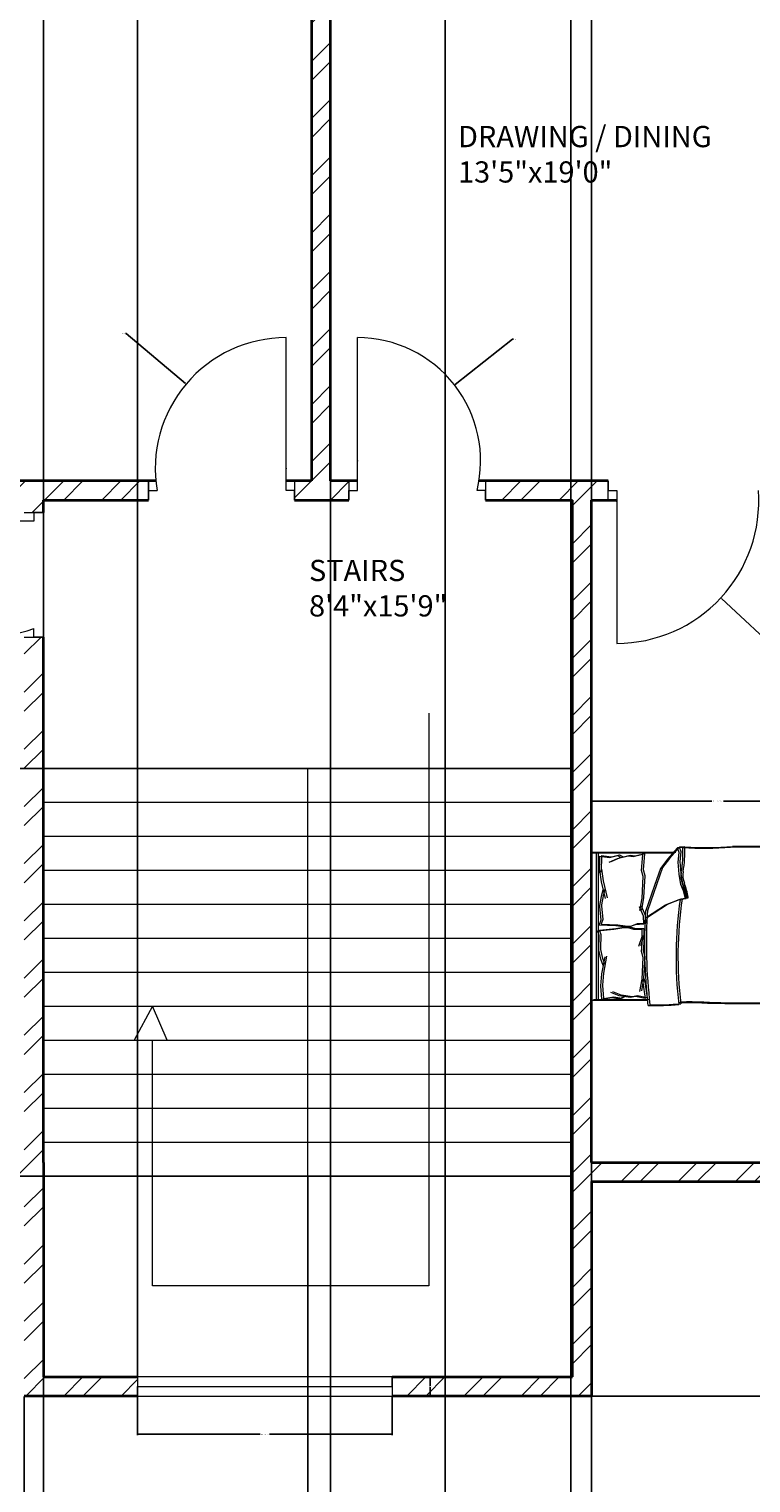
# Model space of a CAD drawing. Units: inches. Extents: x 2064 to 2782, y 1196 to 2299.
# Tile 4 of 11: x 2320 to 2490, y 1620 to 1963. Entities that reach past the tile are written whole.
import ezdxf

# ---------------------------------------------------------------- set-up
doc = ezdxf.new("R2010")
doc.units = ezdxf.units.IN
for name, color, linetype, lineweight in [('A-ANNO-DIMS', 2, 'Continuous', 18), ('A-AREA-IDEN', 7, 'Continuous', 18), ('A-DOOR', 11, 'Continuous', 18), ('A-FLOR-STRS', 81, 'Continuous', 18), ('A-FURN', 8, 'Continuous', 13), ('A-GLAZ', 151, 'Continuous', 18), ('A-WALL', 7, 'Continuous', 35), ('A-WALL-PATT', 9, 'Continuous', 13)]:
    doc.layers.add(name, color=color, linetype=linetype, lineweight=lineweight)
doc.styles.get("Standard").update_dxf_attribs({"font": 'arial.ttf'})
doc.dimstyles.get("Standard").update_dxf_attribs({"dimtxt": 0.18, "dimasz": 0.18, "dimexe": 0.18, "dimexo": 0.0625, "dimgap": 0.09, "dimtad": 0, "dimtih": 1, "dimtoh": 1, "dimdec": 4, "dimzin": 0, "dimdsep": 46, "dimtxsty": 'Standard', "dimcen": 0.09, "dimadec": 0, "dimazin": 0, "dimtfac": 1, "dimtdec": 4, "dimtofl": 0, "dimtmove": 0, "dimatfit": 3, "dimfxl": 1, "dimtolj": 1, "dimtzin": 0, "dimarcsym": 0})

# ---------------------------------------------------------------- blocks, each defined once
blk = doc.blocks.new('BED-DOUBLE')
for p, q in [((2.53, 46.14), (2.53, 59.33)), ((2.53, 46.14), (2.53, 59.33)), ((2.53, 59.33), (37.35, 59.33)), ((2.53, 58.22), (37.35, 58.22)), ((2.53, 58.22), (37.35, 58.22)), ((2.7, 45.67), (2.7, 58.87)), ((2.7, 45.67), (2.7, 58.87)), ((37.35, 59.33), (37.35, 39.95)), ((37.35, 59.33), (37.35, 39.95)), ((37.52, 59.33), (37.52, 58.87)), ((37.52, 58.87), (37.52, 39.48)), ((37.52, 58.87), (37.52, 39.48)), ((2.7, 57.75), (37.52, 57.75)), ((2.7, 57.75), (37.52, 57.75)), ((2.84, 56.9), (5.96, 57.14)), ((2.84, 56.9), (5.96, 57.14)), ((2.84, 56.92), (3.26, 54.6)), ((2.84, 56.92), (3.26, 54.6)), ((3, 56.45), (3.43, 54.14)), ((3, 56.45), (3.43, 54.14)), ((3.01, 56.44), (6.13, 56.68)), ((3.01, 56.44), (6.13, 56.68)), ((3.68, 52.81), (4.42, 54.81)), ((3.68, 52.81), (4.42, 54.81)), ((5.96, 57.14), (6.04, 57.13)), ((5.96, 57.14), (6.04, 57.13)), ((6.04, 57.13), (8.82, 56.92)), ((6.04, 57.13), (8.82, 56.92)), ((6.13, 56.68), (6.2, 56.66)), ((6.13, 56.68), (6.2, 56.66)), ((6.2, 56.66), (8.99, 56.45)), ((6.2, 56.66), (8.99, 56.45)), ((8.82, 56.92), (12.82, 56.18)), ((8.82, 56.92), (12.82, 56.18)), ((8.99, 56.45), (12.99, 55.72)), ((8.99, 56.45), (12.99, 55.72)), ((10.82, 56.6), (12.3, 57.13)), ((10.82, 56.6), (12.3, 57.13)), ((10.99, 56.14), (12.46, 56.66)), ((10.99, 56.14), (12.46, 56.66)), ((12.3, 57.13), (14.4, 57.66)), ((12.3, 57.13), (14.4, 57.66)), ((12.46, 56.66), (14.57, 57.19)), ((12.46, 56.66), (14.57, 57.19)), ((14.4, 57.66), (14.64, 57.66)), ((14.4, 57.66), (14.64, 57.66)), ((14.57, 57.19), (14.8, 57.19)), ((14.57, 57.19), (14.8, 57.19)), ((14.64, 57.66), (17.88, 57.55)), ((14.64, 57.66), (17.88, 57.55)), ((14.8, 57.19), (18.04, 57.09)), ((14.8, 57.19), (18.04, 57.09)), ((17.88, 57.55), (18.93, 57.97)), ((17.88, 57.55), (18.93, 57.97)), ((18.04, 57.09), (19.1, 57.51)), ((18.04, 57.09), (19.1, 57.51)), ((18.93, 57.97), (19.35, 54.07)), ((18.93, 57.97), (19.35, 54.07)), ((19.1, 57.51), (19.52, 53.61)), ((19.1, 57.51), (19.52, 53.61)), ((20.38, 57.52), (20.2, 53.6)), ((20.38, 57.52), (20.21, 53.6)), ((20.55, 57.05), (20.37, 53.14)), ((20.55, 57.05), (20.37, 53.14)), ((21.46, 57.16), (20.38, 57.52)), ((21.46, 57.16), (20.38, 57.52)), ((21.63, 56.7), (20.55, 57.05)), ((21.63, 56.7), (20.55, 57.05)), ((24.69, 57.47), (21.46, 57.16)), ((24.69, 57.47), (21.46, 57.16)), ((24.85, 57.01), (21.63, 56.7)), ((24.85, 57.01), (21.63, 56.7)), ((24.92, 57.49), (24.69, 57.47)), ((24.92, 57.49), (24.69, 57.47)), ((25.09, 57.02), (24.85, 57.01)), ((25.09, 57.02), (24.85, 57.01)), ((27.05, 57.09), (24.92, 57.49)), ((27.05, 57.09), (24.92, 57.49)), ((27.22, 56.63), (25.09, 57.02)), ((27.22, 56.63), (25.09, 57.02)), ((30.54, 57.1), (26.59, 56.11)), ((30.54, 57.1), (26.59, 56.11)), ((30.7, 56.63), (26.75, 55.65)), ((30.7, 56.63), (26.75, 55.65)), ((28.56, 56.66), (27.05, 57.09)), ((28.56, 56.66), (27.05, 57.09)), ((28.73, 56.19), (27.22, 56.63)), ((28.73, 56.19), (27.22, 56.63)), ((33.3, 57.48), (30.54, 57.1)), ((33.3, 57.48), (30.54, 57.1)), ((33.47, 57.02), (30.7, 56.63)), ((33.47, 57.02), (30.7, 56.63)), ((36.51, 57.47), (32.57, 57.54)), ((32.57, 57.54), (33.3, 57.48)), ((36.51, 57.47), (32.57, 57.54)), ((32.57, 57.54), (33.3, 57.48)), ((36.68, 57.01), (32.74, 57.08)), ((32.74, 57.08), (33.47, 57.02)), ((36.67, 57.01), (32.74, 57.08)), ((32.74, 57.08), (33.47, 57.02)), ((35.92, 53.32), (35.06, 55.27)), ((35.92, 53.32), (35.06, 55.27)), ((36.09, 52.85), (35.23, 54.8)), ((36.09, 52.85), (35.23, 54.8)), ((36.51, 57.47), (36.23, 55.13)), ((36.51, 57.47), (36.23, 55.13)), ((36.23, 55.13), (36.67, 53.26)), ((36.23, 55.13), (36.67, 53.26)), ((36.68, 57.01), (36.4, 54.67)), ((36.67, 57.01), (36.4, 54.67)), ((3.26, 54.6), (2.94, 52.71)), ((3.26, 54.6), (2.94, 52.71)), ((2.94, 52.71), (3.36, 51.97)), ((2.94, 52.71), (3.36, 51.97)), ((3.43, 54.14), (3.11, 52.24)), ((3.43, 54.14), (3.11, 52.24)), ((3.11, 52.24), (3.53, 51.5)), ((3.11, 52.24), (3.53, 51.5)), ((3.26, 50.18), (3.68, 52.81)), ((3.26, 50.18), (3.68, 52.81)), ((3.43, 49.71), (3.85, 52.34)), ((3.43, 49.71), (3.85, 52.34)), ((3.85, 52.34), (4.58, 54.35)), ((3.85, 52.34), (4.58, 54.35)), ((19.35, 54.07), (19.77, 51.76)), ((19.35, 54.07), (19.77, 51.76)), ((19.52, 53.61), (19.94, 51.29)), ((19.52, 53.61), (19.94, 51.29)), ((19.77, 51.76), (19.77, 50.81)), ((19.77, 51.76), (19.77, 50.81)), ((20.21, 53.6), (19.93, 51.26)), ((20.2, 53.6), (19.93, 51.26)), ((20.37, 53.14), (20.1, 50.8)), ((20.37, 53.14), (20.1, 50.8)), ((36.51, 50.72), (35.92, 53.32)), ((36.51, 50.72), (35.92, 53.32)), ((36.68, 50.25), (36.09, 52.85)), ((36.67, 50.25), (36.09, 52.85)), ((36.67, 53.26), (36.29, 52.5)), ((36.67, 53.26), (36.29, 52.5)), ((36.4, 54.67), (36.83, 52.79)), ((36.4, 54.67), (36.83, 52.79)), ((36.83, 52.79), (36.46, 52.03)), ((36.83, 52.79), (36.46, 52.03)), ((3.05, 46.7), (3.47, 49.02)), ((3.05, 46.7), (3.47, 49.02)), ((3.21, 46.24), (3.64, 48.55)), ((3.21, 46.24), (3.64, 48.55)), ((3.47, 49.02), (3.26, 50.18)), ((3.47, 49.02), (3.26, 50.18)), ((3.64, 48.55), (3.43, 49.71)), ((3.64, 48.55), (3.43, 49.71)), ((4.65, 47.95), (7.59, 47.46)), ((4.65, 47.95), (7.59, 47.46)), ((17.56, 47.49), (15.27, 48.28)), ((17.56, 47.49), (15.27, 48.28)), ((19.77, 50.81), (19.35, 49.44)), ((19.77, 50.81), (19.35, 49.44)), ((19.35, 49.44), (19.35, 47.49)), ((19.35, 49.44), (19.35, 47.49)), ((19.94, 50.34), (19.52, 48.97)), ((19.94, 50.34), (19.52, 48.97)), ((19.52, 48.97), (19.52, 47.02)), ((19.52, 48.97), (19.52, 47.02)), ((19.93, 51.26), (19.99, 50.32)), ((19.93, 51.26), (19.99, 50.32)), ((19.94, 51.29), (19.94, 50.34)), ((19.94, 51.29), (19.94, 50.34)), ((19.99, 50.32), (20.49, 48.98)), ((19.99, 50.32), (20.49, 48.98)), ((20.1, 50.8), (20.15, 49.85)), ((20.1, 50.8), (20.15, 49.85)), ((20.15, 49.85), (20.66, 48.51)), ((20.15, 49.85), (20.66, 48.51)), ((20.49, 48.98), (20.62, 47.03)), ((20.49, 48.98), (20.62, 47.03)), ((20.66, 48.51), (20.78, 46.56)), ((20.66, 48.51), (20.78, 46.56)), ((22.4, 47.14), (24.64, 48.08)), ((22.4, 47.14), (24.64, 48.08)), ((23.72, 47.95), (26.66, 47.46)), ((23.72, 47.95), (26.66, 47.46)), ((36.37, 49.55), (36.51, 50.72)), ((36.37, 49.55), (36.51, 50.72)), ((36.94, 47.26), (36.37, 49.55)), ((36.94, 47.26), (36.37, 49.55)), ((36.54, 49.08), (36.68, 50.25)), ((36.54, 49.08), (36.67, 50.25)), ((37.1, 46.79), (36.54, 49.08)), ((37.1, 46.79), (36.54, 49.08)), ((6.76, 47.23), (3.05, 46.7)), ((6.76, 47.23), (3.05, 46.7)), ((6.93, 46.76), (3.21, 46.24)), ((6.93, 46.76), (3.21, 46.24)), ((4.82, 47.48), (7.75, 47)), ((4.82, 47.48), (7.75, 47)), ((7.59, 47.46), (6.76, 47.23)), ((7.59, 47.46), (6.76, 47.23)), ((7.75, 47), (6.93, 46.76)), ((7.75, 47), (6.93, 46.76)), ((7.59, 47.46), (12.69, 47.15)), ((7.59, 47.46), (12.69, 47.15)), ((7.75, 47), (12.86, 46.68)), ((7.75, 47), (12.86, 46.68)), ((12.69, 47.15), (14.12, 47.55)), ((12.69, 47.15), (14.12, 47.55)), ((12.86, 46.68), (14.29, 47.09)), ((12.86, 46.68), (14.29, 47.09)), ((14.12, 47.55), (17.86, 47.26)), ((14.12, 47.55), (17.86, 47.26)), ((14.29, 47.09), (18.03, 46.79)), ((14.29, 47.09), (18.03, 46.79)), ((17.73, 47.02), (15.44, 47.82)), ((17.73, 47.02), (15.44, 47.82)), ((19.35, 47.49), (17.56, 47.49)), ((19.35, 47.49), (17.56, 47.49)), ((19.52, 47.02), (17.73, 47.02)), ((19.52, 47.02), (17.73, 47.02)), ((20.62, 47.03), (22.4, 47.14)), ((20.62, 47.03), (22.4, 47.14)), ((20.78, 46.56), (22.57, 46.67)), ((20.78, 46.56), (22.57, 46.67)), ((22.05, 46.67), (25.1, 41.94)), ((22.05, 46.67), (25.1, 41.94)), ((22.21, 46.2), (25.26, 41.47)), ((22.21, 46.2), (25.26, 41.47)), ((22.57, 46.67), (24.81, 47.61)), ((22.57, 46.67), (24.81, 47.61)), ((29.61, 44.53), (23.54, 46.67)), ((29.61, 44.53), (23.54, 46.67)), ((29.78, 44.07), (23.7, 46.2)), ((29.78, 44.07), (23.7, 46.2)), ((23.89, 47.48), (26.83, 47)), ((23.89, 47.48), (26.83, 47)), ((26.66, 47.46), (31.77, 47.15)), ((26.66, 47.46), (31.77, 47.15)), ((26.83, 47), (31.94, 46.68)), ((26.83, 47), (31.94, 46.68)), ((33.67, 43.07), (29.61, 44.53)), ((33.67, 43.07), (29.61, 44.53)), ((31.77, 47.15), (33.2, 47.55)), ((31.77, 47.15), (33.2, 47.55)), ((31.94, 46.68), (33.36, 47.09)), ((31.94, 46.68), (33.36, 47.09)), ((33.2, 47.55), (36.94, 47.26)), ((33.2, 47.55), (36.94, 47.26)), ((33.36, 47.09), (37.1, 46.79)), ((33.36, 47.09), (37.1, 46.79)), ((25.1, 41.94), (26.34, 38.67)), ((25.1, 41.94), (26.34, 38.67)), ((25.26, 41.47), (26.51, 38.2)), ((25.26, 41.47), (26.51, 38.2)), ((33.84, 42.6), (29.78, 44.07)), ((33.84, 42.6), (29.78, 44.07)), ((35.82, 41.49), (33.67, 43.07)), ((35.82, 41.49), (33.67, 43.07)), ((35.98, 41.02), (33.84, 42.6)), ((35.98, 41.02), (33.84, 42.6)), ((38.52, 39.12), (35.82, 41.49)), ((38.52, 39.12), (35.82, 41.49)), ((26.34, 38.67), (26.56, 37.2)), ((26.34, 38.67), (26.56, 37.2)), ((26.51, 38.2), (26.73, 36.74)), ((26.51, 38.2), (26.73, 36.74)), ((28.37, 37.65), (29.84, 38.33)), ((28.37, 37.65), (29.84, 38.33)), ((28.54, 37.19), (30, 37.87)), ((28.54, 37.19), (30, 37.87)), ((29.84, 38.33), (32.32, 38.67)), ((29.84, 38.33), (32.32, 38.67)), ((30, 37.87), (32.49, 38.2)), ((30, 37.87), (32.49, 38.2)), ((32.32, 38.67), (35.14, 38.9)), ((32.32, 38.67), (35.14, 38.9)), ((32.49, 38.2), (35.31, 38.43)), ((32.49, 38.2), (35.31, 38.43)), ((35.14, 38.9), (37.4, 38.67)), ((35.14, 38.9), (37.4, 38.67)), ((35.31, 38.43), (37.56, 38.2)), ((35.31, 38.43), (37.56, 38.2)), ((38.68, 38.65), (35.98, 41.02)), ((38.68, 38.65), (35.98, 41.02)), ((37.4, 38.67), (38.52, 39.12)), ((37.4, 38.67), (38.52, 39.12)), ((37.56, 38.2), (38.68, 38.65)), ((37.56, 38.2), (38.68, 38.65)), ((38.57, 37.85), (38.52, 39.12, 2.82)), ((38.57, 37.85), (38.52, 39.12, 2.82)), ((38.74, 37.38), (38.68, 38.65, 2.82)), ((38.74, 37.38), (38.68, 38.65, 2.82)), ((26.56, 37.2), (28.37, 37.65)), ((26.56, 37.2), (28.37, 37.65)), ((26.73, 36.74), (28.54, 37.19)), ((26.73, 36.74), (28.54, 37.19)), ((10.97, 1.6), (28.91, 1.6)), ((10.97, 1.6), (28.91, 1.6)), ((11.14, 1.14), (29.07, 1.14)), ((11.14, 1.14), (29.07, 1.14))]:
    blk.add_line(p, q)
for centre, radius, start, end in [((62.04, 44.69), 60.69, 178.7218, 185.604), ((62.04, 44.69), 60.69, 178.7218, 185.604), ((15.56, -73.3), 120.19, 86.0865, 96.7821), ((15.56, -73.3), 120.19, 86.0865, 96.7821), ((62.21, 44.23), 60.69, 178.7218, 185.604), ((62.21, 44.23), 60.69, 178.7218, 185.604), ((15.73, -73.76), 120.19, 86.0865, 96.7821), ((15.73, -73.76), 120.19, 86.0865, 96.7821), ((12.94, -54.55), 94, 81.7845, 96.9006), ((12.94, -54.55), 94, 81.7845, 96.9006), ((13.1, -55.01), 94, 81.7845, 96.9006), ((13.1, -55.01), 94, 81.7845, 96.9006), ((-121.89, 36.62), 123.93, 358.4762, 1.0082), ((-121.89, 36.62), 123.93, 358.4762, 1.0082), ((-121.72, 36.16), 123.93, 358.4762, 1.0082), ((-121.72, 36.16), 123.93, 358.4762, 1.0082), ((22.7, 58.25), 21.6, 280.6617, 289.8806), ((22.7, 58.25), 21.6, 280.6617, 289.8806), ((31.87, 33.79), 4.53, 78.6608, 113.7384), ((31.87, 33.79), 4.53, 78.6608, 113.7384), ((32.04, 33.32), 4.53, 78.6608, 113.7384), ((32.04, 33.32), 4.53, 78.6608, 113.7384), ((37.39, 64.18), 26.36, 259.8763, 272.5657), ((37.39, 64.18), 26.36, 259.8763, 272.5657), ((37.56, 63.72), 26.36, 259.8763, 272.5657), ((37.56, 63.72), 26.36, 259.8763, 272.5657), ((132.79, 32.88), 94.35, 176.9791, 183.8365), ((132.79, 32.88), 94.35, 176.9791, 183.8365), ((26.69, 37.16), 0.134, 160.2464, 271.1377), ((26.69, 37.16), 0.134, 160.2464, 271.1377), ((26.86, 36.69), 0.134, 160.2464, 271.1377), ((26.86, 36.69), 0.134, 160.2464, 271.1377), ((22.86, 57.79), 21.6, 280.6617, 289.8806), ((22.86, 57.79), 21.6, 280.6617, 289.8806), ((132.95, 32.41), 94.35, 176.9791, 183.8365), ((132.95, 32.41), 94.35, 176.9791, 183.8365), ((353.21, 22.46), 351.38, 178.2277, 181.7185), ((353.21, 22.46), 351.38, 178.2277, 181.7185), ((353.38, 21.99), 351.38, 178.2277, 181.7185), ((353.38, 21.99), 351.38, 178.2277, 181.7185), ((-3284.8, 9.92), 3323.5, 0.00217, 0.28689), ((-3284.8, 9.92), 3323.5, 0.00217, 0.28689), ((-3284.64, 9.46), 3323.5, 0.00217, 0.28689), ((-3284.64, 9.46), 3323.5, 0.00217, 0.28689), ((-19.6, 12.33), 21.59, 346.0648, 358.9113), ((-19.6, 12.33), 21.59, 346.0648, 358.9113), ((-19.43, 11.87), 21.59, 346.0648, 358.9113), ((-19.43, 11.87), 21.59, 346.0648, 358.9113), ((-15.78, 8.14), 17.17, 337.9751, 356.652), ((-15.78, 8.14), 17.17, 337.9751, 356.652), ((55.48, 9.31), 16.8, 177.4714, 206.4681), ((55.48, 9.31), 16.8, 177.4714, 206.4681), ((55.65, 8.84), 16.8, 177.4714, 206.4681), ((55.65, 8.84), 16.8, 177.4714, 206.4681), ((-15.61, 7.67), 17.17, 337.9751, 356.652), ((-15.61, 7.67), 17.17, 337.9751, 356.652), ((0.79, 1.26), 0.793, 146.1736, 293.4781), ((0.79, 1.26), 0.793, 146.1736, 293.4781), ((0.96, 0.79), 0.793, 146.1736, 293.4781), ((0.96, 0.79), 0.793, 146.1736, 293.4781), ((15.61, -86.98), 88.71, 92.9958, 99.4091), ((15.61, -86.98), 88.71, 92.9958, 99.4091), ((15.78, -87.45), 88.71, 92.9958, 99.4091), ((15.78, -87.45), 88.71, 92.9958, 99.4091), ((-12.55, 76.61), 77.56, 283.3832, 287.7053), ((-12.55, 76.61), 77.56, 283.3832, 287.7053), ((-12.38, 76.14), 77.56, 283.3832, 287.7053), ((-12.38, 76.14), 77.56, 283.3832, 287.7053), ((29.98, -95.32), 96.92, 84.4998, 90.6351), ((29.98, -95.32), 96.92, 84.4998, 90.6351), ((30.15, -95.78), 96.92, 84.4998, 90.6351), ((30.15, -95.78), 96.92, 84.4998, 90.6351), ((39.64, 1.87), 0.803, 242.6588, 356.02), ((39.64, 1.87), 0.803, 242.6588, 356.02), ((39.81, 1.41), 0.803, 242.6588, 356.02), ((39.81, 1.41), 0.803, 242.6588, 356.02)]:
    blk.add_arc(centre, radius, start, end)
blk = doc.blocks.new('WIN-60IN')
for p, q in [((0, 4.5), (0, 0)), ((60, 4.5), (0, 4.5)), ((60, 2.25), (60, 4.5)), ((60, 4.5), (60, 0)), ((0, 0), (0, 2.25)), ((0, 2.25), (60, 2.25)), ((0, 0), (60, 0))]:
    blk.add_line(p, q)
blk = doc.blocks.new('*D8')
at = {"layer": 'A-ANNO-DIMS', "color": 0, "lineweight": -2, "transparency": 16777216}
for p, q in [((2452.17, 1772.06), (2452.17, 1781.09)), ((2452.35, 1780.91), (2480.51, 1780.91)), ((2511.4, 1780.91), (2483.24, 1780.91)), ((2511.58, 1772.06), (2511.58, 1781.09))]:
    blk.add_line(p, q, dxfattribs=at)
at = {"layer": 'A-ANNO-DIMS', "color": 0, "transparency": 16777216}
for points in [[(2452.35, 1780.94), (2452.35, 1780.88), (2452.17, 1780.91)], [(2511.4, 1780.94), (2511.4, 1780.88), (2511.58, 1780.91)]]:
    blk.add_solid(points, dxfattribs=at)
at = {"layer": 'Defpoints', "color": 0, "transparency": 16777216}
for p in [(2452.17, 1780.91), (2452.17, 1771.99), (2511.58, 1771.99)]:
    blk.add_point(p, dxfattribs=at)
at = {"layer": 'A-ANNO-DIMS', "color": 0, "transparency": 16777216, "insert": (2481.87, 1780.91), "char_height": 0.18, "attachment_point": 5}
blk.add_mtext('\\A1;DOUBLE BED 59 TYP.', dxfattribs=at)
blk = doc.blocks.new('*D10')
at = {"layer": 'A-ANNO-DIMS', "color": 0, "lineweight": -2, "transparency": 16777216}
for p, q in [((2345.15, 1640.73), (2345.15, 1631.61)), ((2405.15, 1640.73), (2405.15, 1631.61)), ((2345.33, 1631.79), (2374.03, 1631.79)), ((2404.97, 1631.79), (2376.27, 1631.79))]:
    blk.add_line(p, q, dxfattribs=at)
at = {"layer": 'A-ANNO-DIMS', "color": 0, "transparency": 16777216}
for points in [[(2345.33, 1631.82), (2345.33, 1631.76), (2345.15, 1631.79)], [(2404.97, 1631.82), (2404.97, 1631.76), (2405.15, 1631.79)]]:
    blk.add_solid(points, dxfattribs=at)
at = {"layer": 'Defpoints', "color": 0, "transparency": 16777216}
for p in [(2345.15, 1640.79), (2405.15, 1640.79), (2405.15, 1631.79)]:
    blk.add_point(p, dxfattribs=at)
at = {"layer": 'A-ANNO-DIMS', "color": 0, "transparency": 16777216, "insert": (2375.15, 1631.79), "char_height": 0.18, "attachment_point": 5}
blk.add_mtext('\\A1;WINDOW 60 TYP.', dxfattribs=at)
blk = doc.blocks.new('*D11')
at = {"layer": 'A-ANNO-DIMS', "color": 0, "lineweight": -2, "transparency": 16777216}
for p, q in [((2405.21, 1645.29), (2414.33, 1645.29)), ((2414.15, 1645.11), (2414.15, 1643.22)), ((2405.21, 1640.79), (2414.33, 1640.79)), ((2414.15, 1640.97), (2414.15, 1642.86))]:
    blk.add_line(p, q, dxfattribs=at)
at = {"layer": 'A-ANNO-DIMS', "color": 0, "transparency": 16777216}
for points in [[(2414.12, 1645.11), (2414.18, 1645.11), (2414.15, 1645.29)], [(2414.12, 1640.97), (2414.18, 1640.97), (2414.15, 1640.79)]]:
    blk.add_solid(points, dxfattribs=at)
at = {"layer": 'Defpoints', "color": 0, "transparency": 16777216}
for p in [(2405.15, 1645.29), (2414.15, 1645.29), (2405.15, 1640.79)]:
    blk.add_point(p, dxfattribs=at)
at = {"layer": 'A-ANNO-DIMS', "color": 0, "transparency": 16777216, "insert": (2414.15, 1643.04), "char_height": 0.18, "attachment_point": 5}
blk.add_mtext('\\A1;5 TYP.', dxfattribs=at)
blk = doc.blocks.new('*D23')
at = {"layer": 'A-ANNO-DIMS', "color": 0, "lineweight": -2, "transparency": 16777216}
for p, q in [((2653.23, 2234.29), (2688.85, 2234.29)), ((2688.67, 2234.11), (2688.67, 1937.72)), ((2688.67, 1640.97), (2688.67, 1937.36)), ((2452.23, 1640.79), (2688.85, 1640.79))]:
    blk.add_line(p, q, dxfattribs=at)
at = {"layer": 'A-ANNO-DIMS', "color": 0, "transparency": 16777216}
for points in [[(2688.64, 2234.11), (2688.7, 2234.11), (2688.67, 2234.29)], [(2688.64, 1640.97), (2688.7, 1640.97), (2688.67, 1640.79)]]:
    blk.add_solid(points, dxfattribs=at)
at = {"layer": 'Defpoints', "color": 0, "transparency": 16777216}
for p in [(2653.17, 2234.29), (2688.67, 2234.29), (2452.17, 1640.79)]:
    blk.add_point(p, dxfattribs=at)
at = {"layer": 'A-ANNO-DIMS', "color": 0, "transparency": 16777216, "insert": (2688.67, 1937.54), "char_height": 0.18, "attachment_point": 5}
blk.add_mtext('\\A1;593.5', dxfattribs=at)
blk = doc.blocks.new('*D25')
at = {"layer": 'A-ANNO-DIMS', "color": 0, "lineweight": -2, "transparency": 16777216}
for p, q in [((2318.45, 1640.73), (2318.45, 1539.01)), ((2452.17, 1640.73), (2452.17, 1539.01)), ((2318.63, 1539.19), (2384.86, 1539.19)), ((2451.99, 1539.19), (2385.77, 1539.19))]:
    blk.add_line(p, q, dxfattribs=at)
at = {"layer": 'A-ANNO-DIMS', "color": 0, "transparency": 16777216}
for points in [[(2318.63, 1539.22), (2318.63, 1539.16), (2318.45, 1539.19)], [(2451.99, 1539.22), (2451.99, 1539.16), (2452.17, 1539.19)]]:
    blk.add_solid(points, dxfattribs=at)
at = {"layer": 'Defpoints', "color": 0, "transparency": 16777216}
for p in [(2318.45, 1640.79), (2452.17, 1640.79), (2452.17, 1539.19)]:
    blk.add_point(p, dxfattribs=at)
at = {"layer": 'A-ANNO-DIMS', "color": 0, "transparency": 16777216, "insert": (2385.31, 1539.19), "char_height": 0.18, "attachment_point": 5}
blk.add_mtext('\\A1;133.72', dxfattribs=at)
blk = doc.blocks.new('*D27')
at = {"layer": 'A-ANNO-DIMS', "color": 0, "lineweight": -2, "transparency": 16777216}
for p, q in [((2452.17, 1640.85), (2452.17, 2269.97)), ((2452.35, 2269.79), (2493.09, 2269.79)), ((2534.61, 2269.79), (2493.87, 2269.79)), ((2534.79, 1643.35), (2534.79, 2269.97))]:
    blk.add_line(p, q, dxfattribs=at)
at = {"layer": 'A-ANNO-DIMS', "color": 0, "transparency": 16777216}
for points in [[(2452.35, 2269.82), (2452.35, 2269.76), (2452.17, 2269.79)], [(2534.61, 2269.82), (2534.61, 2269.76), (2534.79, 2269.79)]]:
    blk.add_solid(points, dxfattribs=at)
at = {"layer": 'Defpoints', "color": 0, "transparency": 16777216}
for p in [(2534.79, 2269.79), (2534.79, 1643.29), (2452.17, 1640.79)]:
    blk.add_point(p, dxfattribs=at)
at = {"layer": 'A-ANNO-DIMS', "color": 0, "transparency": 16777216, "insert": (2493.48, 2269.79), "char_height": 0.18, "attachment_point": 5}
blk.add_mtext('\\A1;82.62', dxfattribs=at)
blk = doc.blocks.new('*D35')
at = {"layer": 'A-ANNO-DIMS', "color": 0, "lineweight": -2, "transparency": 16777216}
for p, q in [((2309.4, 1932.85), (2309.4, 2269.97)), ((2309.58, 2269.79), (2347.37, 2269.79)), ((2385.94, 2269.79), (2348.16, 2269.79)), ((2386.12, 1856.35), (2386.12, 2269.97))]:
    blk.add_line(p, q, dxfattribs=at)
at = {"layer": 'A-ANNO-DIMS', "color": 0, "transparency": 16777216}
for points in [[(2309.58, 2269.82), (2309.58, 2269.76), (2309.4, 2269.79)], [(2385.94, 2269.82), (2385.94, 2269.76), (2386.12, 2269.79)]]:
    blk.add_solid(points, dxfattribs=at)
at = {"layer": 'Defpoints', "color": 0, "transparency": 16777216}
for p in [(2386.12, 2269.79), (2309.4, 1932.79), (2386.12, 1856.29)]:
    blk.add_point(p, dxfattribs=at)
at = {"layer": 'A-ANNO-DIMS', "color": 0, "transparency": 16777216, "insert": (2347.76, 2269.79), "char_height": 0.18, "attachment_point": 5}
blk.add_mtext('\\A1;76.72', dxfattribs=at)
blk = doc.blocks.new('*D36')
at = {"layer": 'A-ANNO-DIMS', "color": 0, "lineweight": -2, "transparency": 16777216}
for p, q in [((2390.62, 2058.73), (2390.62, 1539.01)), ((2541.17, 2058.73), (2541.17, 1539.01)), ((2390.8, 1539.19), (2465.44, 1539.19)), ((2540.99, 1539.19), (2466.35, 1539.19))]:
    blk.add_line(p, q, dxfattribs=at)
at = {"layer": 'A-ANNO-DIMS', "color": 0, "transparency": 16777216}
for points in [[(2390.8, 1539.22), (2390.8, 1539.16), (2390.62, 1539.19)], [(2540.99, 1539.22), (2540.99, 1539.16), (2541.17, 1539.19)]]:
    blk.add_solid(points, dxfattribs=at)
at = {"layer": 'Defpoints', "color": 0, "transparency": 16777216}
for p in [(2390.62, 2058.79), (2541.17, 2058.79), (2541.17, 1539.19)]:
    blk.add_point(p, dxfattribs=at)
at = {"layer": 'A-ANNO-DIMS', "color": 0, "transparency": 16777216, "insert": (2465.9, 1539.19), "char_height": 0.18, "attachment_point": 5}
blk.add_mtext('\\A1;150.55', dxfattribs=at)
blk = doc.blocks.new('*D37')
at = {"layer": 'A-ANNO-DIMS', "color": 0, "lineweight": -2, "transparency": 16777216}
for p, q in [((2447.61, 1788.61), (2092.49, 1788.61)), ((2092.67, 1788.43), (2092.67, 1740.79)), ((2092.67, 1692.79), (2092.67, 1740.43)), ((2447.61, 1692.61), (2092.49, 1692.61))]:
    blk.add_line(p, q, dxfattribs=at)
at = {"layer": 'A-ANNO-DIMS', "color": 0, "transparency": 16777216}
for points in [[(2092.64, 1788.43), (2092.7, 1788.43), (2092.67, 1788.61)], [(2092.64, 1692.79), (2092.7, 1692.79), (2092.67, 1692.61)]]:
    blk.add_solid(points, dxfattribs=at)
at = {"layer": 'Defpoints', "color": 0, "transparency": 16777216}
for p in [(2092.67, 1788.61), (2447.67, 1788.61), (2447.67, 1692.61)]:
    blk.add_point(p, dxfattribs=at)
at = {"layer": 'A-ANNO-DIMS', "color": 0, "transparency": 16777216, "insert": (2092.67, 1740.61), "char_height": 0.18, "attachment_point": 5}
blk.add_mtext('\\A1;96', dxfattribs=at)
blk = doc.blocks.new('*D38')
at = {"layer": 'A-ANNO-DIMS', "color": 0, "lineweight": -2, "transparency": 16777216}
for p, q in [((2322.95, 1692.55), (2322.95, 1539.01)), ((2385.31, 1692.55), (2385.31, 1539.01)), ((2323.13, 1539.19), (2353.74, 1539.19)), ((2385.13, 1539.19), (2354.53, 1539.19))]:
    blk.add_line(p, q, dxfattribs=at)
at = {"layer": 'A-ANNO-DIMS', "color": 0, "transparency": 16777216}
for points in [[(2323.13, 1539.22), (2323.13, 1539.16), (2322.95, 1539.19)], [(2385.13, 1539.22), (2385.13, 1539.16), (2385.31, 1539.19)]]:
    blk.add_solid(points, dxfattribs=at)
at = {"layer": 'Defpoints', "color": 0, "transparency": 16777216}
for p in [(2322.95, 1692.61), (2385.31, 1692.61), (2385.31, 1539.19)]:
    blk.add_point(p, dxfattribs=at)
at = {"layer": 'A-ANNO-DIMS', "color": 0, "transparency": 16777216, "insert": (2354.13, 1539.19), "char_height": 0.18, "attachment_point": 5}
blk.add_mtext('\\A1;62.36', dxfattribs=at)
blk = doc.blocks.new('*D39')
at = {"layer": 'A-ANNO-DIMS', "color": 0, "lineweight": -2, "transparency": 16777216}
for p, q in [((2322.95, 1645.35), (2322.95, 2269.97)), ((2323.13, 2269.79), (2333.59, 2269.79)), ((2344.97, 2269.79), (2334.51, 2269.79)), ((2345.15, 1645.35), (2345.15, 2269.97))]:
    blk.add_line(p, q, dxfattribs=at)
at = {"layer": 'A-ANNO-DIMS', "color": 0, "transparency": 16777216}
for points in [[(2323.13, 2269.82), (2323.13, 2269.76), (2322.95, 2269.79)], [(2344.97, 2269.82), (2344.97, 2269.76), (2345.15, 2269.79)]]:
    blk.add_solid(points, dxfattribs=at)
at = {"layer": 'Defpoints', "color": 0, "transparency": 16777216}
for p in [(2345.15, 2269.79), (2322.95, 1645.29), (2345.15, 1645.29)]:
    blk.add_point(p, dxfattribs=at)
at = {"layer": 'A-ANNO-DIMS', "color": 0, "transparency": 16777216, "insert": (2334.05, 2269.79), "char_height": 0.18, "attachment_point": 5}
blk.add_mtext('\\A1;22.194', dxfattribs=at)
blk = doc.blocks.new('*D41')
at = {"layer": 'A-ANNO-DIMS', "color": 0, "lineweight": -2, "transparency": 16777216}
for p, q in [((2417.67, 2229.73), (2417.67, 1539.01)), ((2447.29, 2229.73), (2447.29, 1539.01)), ((2417.85, 1539.19), (2432.08, 1539.19)), ((2447.11, 1539.19), (2432.87, 1539.19))]:
    blk.add_line(p, q, dxfattribs=at)
at = {"layer": 'A-ANNO-DIMS', "color": 0, "transparency": 16777216}
for points in [[(2417.85, 1539.22), (2417.85, 1539.16), (2417.67, 1539.19)], [(2447.11, 1539.22), (2447.11, 1539.16), (2447.29, 1539.19)]]:
    blk.add_solid(points, dxfattribs=at)
at = {"layer": 'Defpoints', "color": 0, "transparency": 16777216}
for p in [(2417.67, 2229.79), (2447.29, 2229.79), (2447.29, 1539.19)]:
    blk.add_point(p, dxfattribs=at)
at = {"layer": 'A-ANNO-DIMS', "color": 0, "transparency": 16777216, "insert": (2432.48, 1539.19), "char_height": 0.18, "attachment_point": 5}
blk.add_mtext('\\A1;29.62', dxfattribs=at)
blk = doc.blocks.new('*D42')
at = {"layer": 'A-ANNO-DIMS', "color": 0, "lineweight": -2, "transparency": 16777216}
for p, q in [((2457.99, 1851.52), (2458.17, 1851.52)), ((2458.08, 1851.43), (2458.08, 1851.61)), ((2497.35, 1815.1), (2482.76, 1828.63)), ((2497.53, 1815.1), (2497.35, 1815.1))]:
    blk.add_line(p, q, dxfattribs=at)
at = {"layer": 'A-ANNO-DIMS', "color": 0, "transparency": 16777216}
blk.add_solid([(2482.78, 1828.66), (2482.74, 1828.61), (2482.63, 1828.76)], dxfattribs=at)
at = {"layer": 'Defpoints', "color": 0, "transparency": 16777216}
for p in [(2458.08, 1851.52), (2482.63, 1828.76)]:
    blk.add_point(p, dxfattribs=at)
at = {"layer": 'A-ANNO-DIMS', "color": 0, "transparency": 16777216, "insert": (2498.01, 1815.1), "char_height": 0.18, "attachment_point": 5}
blk.add_mtext('\\A1;R33.48', dxfattribs=at)
blk = doc.blocks.new('*D43')
at = {"layer": 'A-ANNO-DIMS', "color": 0, "lineweight": -2, "transparency": 16777216}
for p, q in [((2342.29, 1891.03), (2342.47, 1891.03)), ((2342.47, 1891.03), (2356.46, 1879.22)), ((2380.07, 1859.21), (2380.25, 1859.21)), ((2380.16, 1859.12), (2380.16, 1859.3))]:
    blk.add_line(p, q, dxfattribs=at)
at = {"layer": 'A-ANNO-DIMS', "color": 0, "transparency": 16777216}
blk.add_solid([(2356.48, 1879.24), (2356.44, 1879.19), (2356.6, 1879.1)], dxfattribs=at)
at = {"layer": 'Defpoints', "color": 0, "transparency": 16777216}
for p in [(2356.6, 1879.1), (2380.16, 1859.21)]:
    blk.add_point(p, dxfattribs=at)
at = {"layer": 'A-ANNO-DIMS', "color": 0, "transparency": 16777216, "insert": (2341.81, 1891.03), "char_height": 0.18, "attachment_point": 5}
blk.add_mtext('\\A1;R30.83', dxfattribs=at)
blk = doc.blocks.new('*D45')
at = {"layer": 'A-ANNO-DIMS', "color": 0, "lineweight": -2, "transparency": 16777216}
for p, q in [((2433.55, 1889.64), (2419.98, 1879.02)), ((2433.73, 1889.64), (2433.55, 1889.64)), ((2396.89, 1861.01), (2397.07, 1861.01)), ((2396.98, 1860.92), (2396.98, 1861.1))]:
    blk.add_line(p, q, dxfattribs=at)
at = {"layer": 'A-ANNO-DIMS', "color": 0, "transparency": 16777216}
blk.add_solid([(2419.96, 1879.04), (2419.99, 1878.99), (2419.83, 1878.91)], dxfattribs=at)
at = {"layer": 'Defpoints', "color": 0, "transparency": 16777216}
for p in [(2419.83, 1878.91), (2396.98, 1861.01)]:
    blk.add_point(p, dxfattribs=at)
at = {"layer": 'A-ANNO-DIMS', "color": 0, "transparency": 16777216, "insert": (2434.21, 1889.64), "char_height": 0.18, "attachment_point": 5}
blk.add_mtext('\\A1;R29.03', dxfattribs=at)

msp = doc.modelspace()

# ---------------------------------------------------------------- hatches: boundary and pattern name
at = {"layer": 'A-WALL-PATT'}
h = msp.add_hatch(dxfattribs=at)
h.set_pattern_fill('ANSI32', color=256)
h.paths.add_polyline_path([(2489.7688, 2189.2917), (2574.5454, 2189.2917), (2574.5454, 2191.5417), (2574.5454, 2193.7917), (2570.6691, 2193.7917), (2570.6691, 2197.3052), (2568.4191, 2197.3052), (2566.1691, 2197.3052), (2566.1691, 2193.7917), (2494.1691, 2193.7917), (2494.1691, 2229.7917), (2523.2441, 2229.7917), (2523.2441, 2234.2917), (2471.2886, 2234.2917), (2471.2886, 2229.7917), (2489.6691, 2229.7917), (2489.6691, 2193.7917), (2417.6691, 2193.7917), (2417.6691, 2197.0632), (2415.4191, 2197.0632), (2413.1691, 2197.0632), (2413.1691, 2193.7917), (2406.8865, 2193.7917), (2406.8865, 2189.2917), (2485.2688, 2189.2917), (2485.2688, 2063.2917), (2369.1629, 2063.2917), (2369.1629, 2058.7917), (2386.1222, 2058.7917), (2386.1222, 1856.2917), (2382.1576, 1856.2917), (2382.1576, 1851.7917), (2394.9764, 1851.7917), (2394.9764, 1854.0417), (2394.9764, 1856.2917), (2390.6222, 1856.2917), (2390.6222, 2058.7917), (2485.2688, 2058.7917), (2493.762, 2058.7917), (2493.762, 2061.0417), (2493.762, 2063.2917), (2489.7688, 2063.2917)])
h.paths.add_polyline_path([(2447.2886, 2234.2917), (2413.1691, 2234.2917), (2413.1691, 2217.3799), (2417.6691, 2217.3799), (2417.6691, 2229.7917), (2447.2886, 2229.7917)], flags=17)
h.paths.add_polyline_path([(2570.6691, 2234.2917), (2547.2441, 2234.2917), (2547.2441, 2229.7917), (2566.1691, 2229.7917), (2566.1691, 2216.5615), (2570.6691, 2216.5615)], flags=17)
h.paths.add_polyline_path([(2653.1691, 2189.2917), (2653.1691, 2193.7917), (2640.8843, 2193.7917), (2640.8843, 2189.2917), (2648.6691, 2189.2917), (2648.6691, 2162.7138), (2653.1691, 2162.7138)])
h.paths.add_polyline_path([(2653.1691, 2102.7138), (2648.6691, 2102.7138), (2648.6691, 2063.2917), (2526.7281, 2063.2917), (2526.7281, 2058.7917), (2541.1691, 2058.7917), (2541.1691, 1993.2917), (2545.6691, 1993.2917), (2545.6691, 1997.7917), (2545.6691, 2058.7917), (2648.6691, 2058.7917), (2648.6691, 2050.1099), (2653.1691, 2050.1099)])
h.paths.add_polyline_path([(2600.6691, 1856.2917), (2493.4607, 1856.2917), (2493.4607, 1851.7917), (2596.1691, 1851.7917), (2596.1691, 1695.7917), (2594.0816, 1695.7917), (2594.0816, 1691.2917), (2614.7905, 1691.2917), (2614.7905, 1645.2917), (2536.7905, 1645.2917), (2536.7905, 1691.2917), (2539.332, 1691.2917), (2539.332, 1693.5417), (2539.332, 1695.7917), (2452.1691, 1695.7917), (2452.1691, 1851.7917), (2456.0775, 1851.7917), (2456.0775, 1856.2917), (2427.1536, 1856.2917), (2427.1536, 1851.7917), (2447.6691, 1851.7917), (2447.6691, 1695.7917), (2447.6691, 1645.2917), (2405.1469, 1645.2917), (2405.1469, 1640.7917), (2452.1691, 1640.7917), (2452.1691, 1645.2917), (2452.1691, 1691.2917), (2534.7905, 1691.2917), (2534.7905, 1645.2917), (2534.7905, 1643.2917), (2614.7905, 1643.2917), (2616.7905, 1643.2917), (2616.7905, 1691.2917), (2622.4029, 1691.2917), (2622.4029, 1693.7143), (2622.4029, 1695.7917), (2600.6691, 1695.7917), (2600.6691, 1779.7917), (2648.6691, 1779.7917), (2648.6691, 1695.7917), (2646.4029, 1695.7917), (2646.4029, 1691.2917), (2653.1691, 1691.2917), (2653.1691, 1906.3508), (2648.6691, 1906.3508), (2648.6691, 1856.2917), (2648.6691, 1784.2917), (2600.6691, 1784.2917)])
h.paths.add_polyline_path([(2322.9532, 1819.5181), (2320.7032, 1819.5181), (2318.4532, 1819.5181), (2318.4532, 1695.7917), (2242.7664, 1695.7917), (2242.7664, 1691.2917), (2318.4532, 1691.2917), (2318.4532, 1640.7917), (2322.9532, 1640.7917), (2345.1469, 1640.7917), (2345.1469, 1643.0417), (2345.1469, 1645.2917), (2322.9532, 1645.2917), (2322.9532, 1691.2917), (2322.9532, 1695.7917)])
h.paths.add_polyline_path([(2166.1825, 1691.2917), (2164.1825, 1691.2917), (2164.1825, 1643.2917), (2166.1825, 1643.2917), (2246.1825, 1643.2917), (2246.1825, 1645.2917), (2246.1825, 1691.2917), (2244.1825, 1691.2917), (2244.1825, 1645.2917), (2166.1825, 1645.2917)])
h.paths.add_polyline_path([(2309.404, 1932.7917), (2204.1691, 1932.7917), (2204.1691, 1960.0962), (2199.6691, 1960.0962), (2199.6691, 1932.7917), (2132.6691, 1932.7917), (2132.6691, 1951.0737), (2128.1691, 1951.0737), (2128.1691, 1910.0412), (2132.6691, 1910.0412), (2132.6691, 1928.2917), (2304.904, 1928.2917), (2304.904, 1856.2917), (2304.904, 1851.7917), (2318.4532, 1851.7917), (2318.4532, 1848.8308), (2322.9532, 1848.8308), (2322.9532, 1851.7917), (2347.7631, 1851.7917), (2347.7631, 1856.2917), (2309.404, 1856.2917)])
h.paths.add_polyline_path([(2132.6691, 2044.9092), (2130.4191, 2044.9092), (2128.1691, 2044.9092), (2128.1691, 1987.0737), (2132.6691, 1987.0737), (2132.6691, 2004.7917), (2199.6691, 2004.7917), (2204.1691, 2004.7917), (2204.1691, 2009.2917), (2132.6691, 2009.2917)])
h.paths.add_polyline_path([(2186.6691, 2195.9329), (2184.4191, 2195.9329), (2184.4191, 2195.8929), (2182.1691, 2195.9329), (2182.1691, 2193.7917), (2128.1691, 2193.7917), (2128.1691, 2181.4967), (2132.6691, 2181.4967), (2132.6691, 2182.7769), (2132.6691, 2189.2917), (2182.1691, 2189.2917), (2182.1691, 2135.2917), (2179.804, 2135.2917), (2179.804, 2130.7917), (2190.215, 2130.7917), (2190.215, 2133.0417), (2190.215, 2135.2917), (2186.6691, 2135.2917)])
h.paths.add_polyline_path([(2340.0628, 2189.2917), (2340.0628, 2191.5417), (2340.0628, 2193.7917), (2335.1691, 2193.7917), (2335.1691, 2234.2917), (2280.6746, 2234.2917), (2280.6746, 2229.7917), (2330.6691, 2229.7917), (2330.6691, 2193.7917), (2330.6691, 2135.2917), (2218.6309, 2135.2917), (2218.6309, 2130.7917), (2330.7688, 2130.7917), (2330.7688, 2008.4023), (2335.2688, 2008.4023), (2335.2688, 2058.7917), (2338.9208, 2058.7917), (2338.9208, 2061.0417), (2338.9208, 2063.2917), (2335.2688, 2063.2917), (2335.2688, 2189.2917)])
h.paths.add_polyline_path([(2220.6746, 2234.2917), (2182.1691, 2234.2917), (2182.1691, 2227.4187), (2186.6691, 2227.4187), (2186.6691, 2229.7917), (2220.6746, 2229.7917), (2220.6746, 2232.0417)])
h.paths.add_polyline_path([(2158.8146, 2135.2917), (2132.6691, 2135.2917), (2132.6691, 2157.4967), (2128.1691, 2157.4967), (2128.1691, 2104.9092), (2132.6691, 2104.9092), (2132.6691, 2130.7917), (2158.8146, 2130.7917), (2158.8146, 2133.0417)])
h.paths.add_polyline_path([(2396.0464, 2062.2045), (2434.8868, 2062.2045), (2434.8868, 2080.8619), (2396.0464, 2080.8619)], flags=24)
h.paths.add_polyline_path([(2196.1396, 1653.3449), (2232.023, 1653.3449), (2232.023, 1672.0022), (2196.1396, 1672.0022)], flags=25)

# ---------------------------------------------------------------- linework, layer by layer
at = {"layer": 'A-DOOR'}
for p, q in [((2380.1576, 1854.0417), (2380.1576, 1890.0417)), ((2396.9764, 1854.0417), (2396.9764, 1890.0417)), ((2347.7631, 1856.2917), (2347.7631, 1851.7917)), ((2347.7631, 1851.7917), (2347.7631, 1856.2917)), ((2382.1576, 1856.2917), (2382.1576, 1851.7917)), ((2394.9764, 1856.2917), (2394.9764, 1851.7917)), ((2427.1536, 1856.2917), (2427.1536, 1851.7917)), ((2456.0775, 1851.7917), (2456.0775, 1856.2917)), ((2456.0775, 1856.2917), (2456.0775, 1854.0417)), ((2347.7631, 1854.0417), (2349.7631, 1854.0417)), ((2382.1576, 1854.0417), (2380.1576, 1854.0417)), ((2382.1576, 1851.7917), (2382.1576, 1854.0417)), ((2394.9764, 1851.7917), (2394.9764, 1854.0417)), ((2394.9764, 1854.0417), (2396.9764, 1854.0417)), ((2427.1536, 1854.0417), (2425.1536, 1854.0417)), ((2427.1536, 1851.7917), (2427.1536, 1854.0417)), ((2456.0775, 1854.0417), (2458.0775, 1854.0417)), ((2458.0775, 1854.0417), (2458.0775, 1818.0417)), ((2318.4532, 1848.8308), (2322.9532, 1848.8308)), ((2322.9532, 1848.8308), (2320.7032, 1848.8308)), ((2320.7032, 1848.8308), (2320.7032, 1846.8308)), ((2320.7032, 1846.8308), (2284.7032, 1846.8308)), ((2320.7032, 1819.5181), (2320.7032, 1821.5181)), ((2318.4532, 1819.5181), (2322.9532, 1819.5181)), ((2322.9532, 1819.5181), (2320.7032, 1819.5181))]:
    msp.add_line(p, q, dxfattribs=at)
for centre, radius, start, end in [((2380.1576, 1859.2108), 30.8309, 90, 189.651729), ((2396.9764, 1861.0145), 29.0272, 346.100588, 90), ((2458.0775, 1851.5199), 33.4783, 270, 4.319874), ((2311.6023, 1846.8308), 26.8991, 180, 289.775476)]:
    msp.add_arc(centre, radius, start, end, dxfattribs=at)
at = {"layer": 'A-FLOR-STRS'}
for p, q in [((2413.7776, 1801.5754), (2413.7776, 1666.7222)), ((2322.9532, 1788.6099), (2447.6691, 1788.6099)), ((2385.3111, 1692.6099), (2385.3111, 1788.6099)), ((2322.9532, 1780.6099), (2447.6691, 1780.6099)), ((2322.9532, 1772.6099), (2447.6691, 1772.6099)), ((2322.9532, 1764.6099), (2447.6691, 1764.6099)), ((2322.9532, 1756.6099), (2447.6691, 1756.6099)), ((2322.9532, 1748.6099), (2447.6691, 1748.6099)), ((2322.9532, 1740.6099), (2447.6691, 1740.6099)), ((2322.9532, 1732.6099), (2447.6691, 1732.6099)), ((2348.6967, 1732.6099), (2344.3174, 1724.6099)), ((2352.1379, 1724.6099), (2348.6967, 1732.6099)), ((2322.9532, 1724.6099), (2447.6691, 1724.6099)), ((2344.3174, 1724.6099), (2352.1379, 1724.6099)), ((2348.6967, 1666.7222), (2348.6967, 1724.6099)), ((2322.9532, 1716.6099), (2447.6691, 1716.6099)), ((2322.9532, 1708.6099), (2447.6691, 1708.6099)), ((2322.9532, 1700.6099), (2447.6691, 1700.6099)), ((2322.9532, 1692.6099), (2447.6691, 1692.6099)), ((2413.7776, 1666.7222), (2348.6967, 1666.7222))]:
    msp.add_line(p, q, dxfattribs=at)
at = {"layer": 'A-WALL'}
for p, q in [((2386.1222, 2058.7917), (2386.1222, 1856.2917)), ((2390.6222, 1856.2917), (2390.6222, 2058.7917)), ((2349.4652, 1856.2917), (2309.404, 1856.2917)), ((2386.1222, 1856.2917), (2380.1576, 1856.2917)), ((2396.9764, 1856.2917), (2390.6222, 1856.2917)), ((2456.0775, 1856.2917), (2425.6167, 1856.2917)), ((2322.9532, 1851.7917), (2347.7631, 1851.7917)), ((2322.9532, 1848.8308), (2322.9532, 1851.7917)), ((2382.1576, 1851.7917), (2394.9764, 1851.7917)), ((2427.1536, 1851.7917), (2447.6691, 1851.7917)), ((2447.6691, 1695.7917), (2447.6691, 1851.7917)), ((2452.1691, 1695.7917), (2452.1691, 1851.7917)), ((2452.1691, 1851.7917), (2458.0775, 1851.7917)), ((2322.9532, 1695.7917), (2322.9532, 1819.5181)), ((2322.9532, 1695.7917), (2322.9532, 1691.2917)), ((2447.6691, 1645.2917), (2447.6691, 1695.7917)), ((2452.1691, 1695.7917), (2539.332, 1695.7917)), ((2322.9532, 1691.2917), (2322.9532, 1645.2917)), ((2452.1691, 1691.2917), (2452.1691, 1645.2917)), ((2452.1691, 1691.2917), (2534.7905, 1691.2917)), ((2322.9532, 1645.2917), (2345.1469, 1645.2917)), ((2405.1469, 1645.2917), (2447.6691, 1645.2917)), ((2452.1691, 1645.2917), (2452.1691, 1640.7917)), ((2322.9532, 1640.7917), (2318.4532, 1640.7917)), ((2345.1469, 1640.7917), (2322.9532, 1640.7917)), ((2452.1691, 1640.7917), (2405.1469, 1640.7917))]:
    msp.add_line(p, q, dxfattribs=at)

# ---------------------------------------------------------------- block references
at = {"layer": 'A-FURN', "rotation": 89.99999983318565}
msp.add_blockref('BED-DOUBLE', (2511.5038, 1731.3857), dxfattribs=at)
at = {"layer": 'A-GLAZ'}
msp.add_blockref('WIN-60IN', (2345.1469, 1640.7917), dxfattribs=at)

# ---------------------------------------------------------------- texts
at = {"layer": 'A-AREA-IDEN', "char_height": 5, "attachment_point": 1}
for s, width, insert in [('DRAWING / DINING \\P13\'5"x19\'0"', 163.465116, (2420.6837, 1939.884)), ('STAIRS\\P8\'4"x15\'9"', 156.921204, (2385.5649, 1837.7113))]:
    msp.add_mtext_dynamic_manual_height_columns(s, width=width, gutter_width=12.5, heights=[0], dxfattribs=dict(at, insert=insert))

# ---------------------------------------------------------------- dimensions: what is measured, and where the dimension line sits
at = {"layer": 'A-ANNO-DIMS'}
for base, p1, p2, override, picture, middle in [((2386.1222, 2269.7917), (2309.404, 1932.7917), (2386.1222, 1856.2917), {"dimdec": 2, "dimlfac": 1, "dimrnd": 0, "dimzin": 0, "dimdsep": 46, "dimlunit": 2}, '*D35', (2347.7631, 2269.7917)), ((2345.1469, 2269.7917), (2322.9532, 1645.2917), (2345.1469, 1645.2917), {"dimdec": 3, "dimlfac": 1, "dimrnd": 0, "dimzin": 0, "dimdsep": 46, "dimlunit": 2}, '*D39', (2334.0501, 2269.7917)), ((2534.7905, 2269.7917), (2452.1691, 1640.7917), (2534.7905, 1643.2917), {"dimdec": 2, "dimlfac": 1, "dimrnd": 0, "dimzin": 0, "dimdsep": 46, "dimlunit": 2}, '*D27', (2493.4798, 2269.7917)), ((2447.2886, 1539.1896), (2417.6691, 2229.7917), (2447.2886, 2229.7917), {"dimdec": 2, "dimlfac": 1, "dimrnd": 0, "dimzin": 0, "dimdsep": 46, "dimlunit": 2}, '*D41', (2432.4788, 1539.1896)), ((2541.1691, 1539.1896), (2390.6222, 2058.7917), (2541.1691, 2058.7917), {"dimdec": 2, "dimlfac": 1, "dimrnd": 0, "dimzin": 0, "dimdsep": 46, "dimlunit": 2}, '*D36', (2465.8957, 1539.1896)), ((2385.3111, 1539.1896), (2322.9532, 1692.6099), (2385.3111, 1692.6099), {"dimdec": 2, "dimlfac": 1, "dimrnd": 0, "dimzin": 0, "dimdsep": 46, "dimlunit": 2}, '*D38', (2354.1322, 1539.1896)), ((2452.1691, 1539.1896), (2318.4532, 1640.7917), (2452.1691, 1640.7917), {"dimdec": 2, "dimlfac": 1, "dimrnd": 0, "dimzin": 0, "dimdsep": 46, "dimlunit": 2}, '*D25', (2385.3112, 1539.1896))]:
    dim = msp.add_linear_dim(base=base, p1=p1, p2=p2, dimstyle='Standard', override=override, dxfattribs=at)
    dim.commit()
    dim.dimension.update_dxf_attribs({"geometry": picture, "text_midpoint": middle})
for base, p1, p2, override, picture, middle in [((2688.6691, 2234.2917), (2452.1691, 1640.7917), (2653.1691, 2234.2917), {"dimdec": 1, "dimlfac": 1, "dimrnd": 0, "dimzin": 0, "dimdsep": 46, "dimlunit": 2}, '*D23', (2688.6691, 1937.5417)), ((2092.6691, 1788.6099), (2447.6691, 1692.6099), (2447.6691, 1788.6099), {"dimdec": 0, "dimlfac": 1, "dimrnd": 0, "dimzin": 0, "dimdsep": 46, "dimlunit": 2}, '*D37', (2092.6691, 1740.6099))]:
    dim = msp.add_linear_dim(base=base, p1=p1, p2=p2, angle=90, dimstyle='Standard', override=override, dxfattribs=at)
    dim.commit()
    dim.dimension.update_dxf_attribs({"geometry": picture, "text_midpoint": middle})
for center, mpoint, picture, middle in [((2380.1576, 1859.2108), (2356.6, 1879.1), '*D43', (2341.8056, 1891.0336)), ((2396.9764, 1861.0145), (2419.8345, 1878.9054), '*D45', (2434.2092, 1889.6399)), ((2458.0775, 1851.5199), (2482.6257, 1828.7563), '*D42', (2498.0146, 1815.0982))]:
    dim = msp.add_radius_dim(center=center, mpoint=mpoint, dimstyle='Standard', override={"dimdec": 2, "dimlfac": 1, "dimrnd": 0, "dimzin": 0, "dimdsep": 46, "dimlunit": 2}, dxfattribs=at)
    dim.commit()
    dim.dimension.update_dxf_attribs({"geometry": picture, "text_midpoint": middle, "dimtype": 164})
for base, p1, p2, angle, text, picture, middle in [((2452.1691, 1780.905), (2511.5806, 1771.9933), (2452.1691, 1771.9933), 180, 'DOUBLE BED <> TYP.', '*D8', (2481.8748, 1780.905)), ((2414.1469050011, 1645.2916736115), (2405.1469050011, 1640.7916736115), (2405.1469050011, 1645.2916736115), 90, '<> TYP.', '*D11', (2414.1469050011, 1643.0416736115))]:
    dim = msp.add_linear_dim(base=base, p1=p1, p2=p2, angle=angle, text=text, dimstyle='Standard', override={"dimdec": 0, "dimlfac": 1, "dimrnd": 0, "dimzin": 0, "dimdsep": 46, "dimlunit": 2}, dxfattribs=at)
    dim.commit()
    dim.dimension.update_dxf_attribs({"geometry": picture, "text_midpoint": middle})
dim = msp.add_linear_dim(base=(2405.1469, 1631.7917), p1=(2345.1469, 1640.7917), p2=(2405.1469, 1640.7917), text='WINDOW <> TYP.', dimstyle='Standard', override={"dimdec": 0, "dimlfac": 1, "dimrnd": 0, "dimzin": 0, "dimdsep": 46, "dimlunit": 2}, dxfattribs=at)
dim.commit()
dim.dimension.update_dxf_attribs({"geometry": '*D10', "text_midpoint": (2375.1469, 1631.7917)})

doc.saveas('drawing.dxf')
